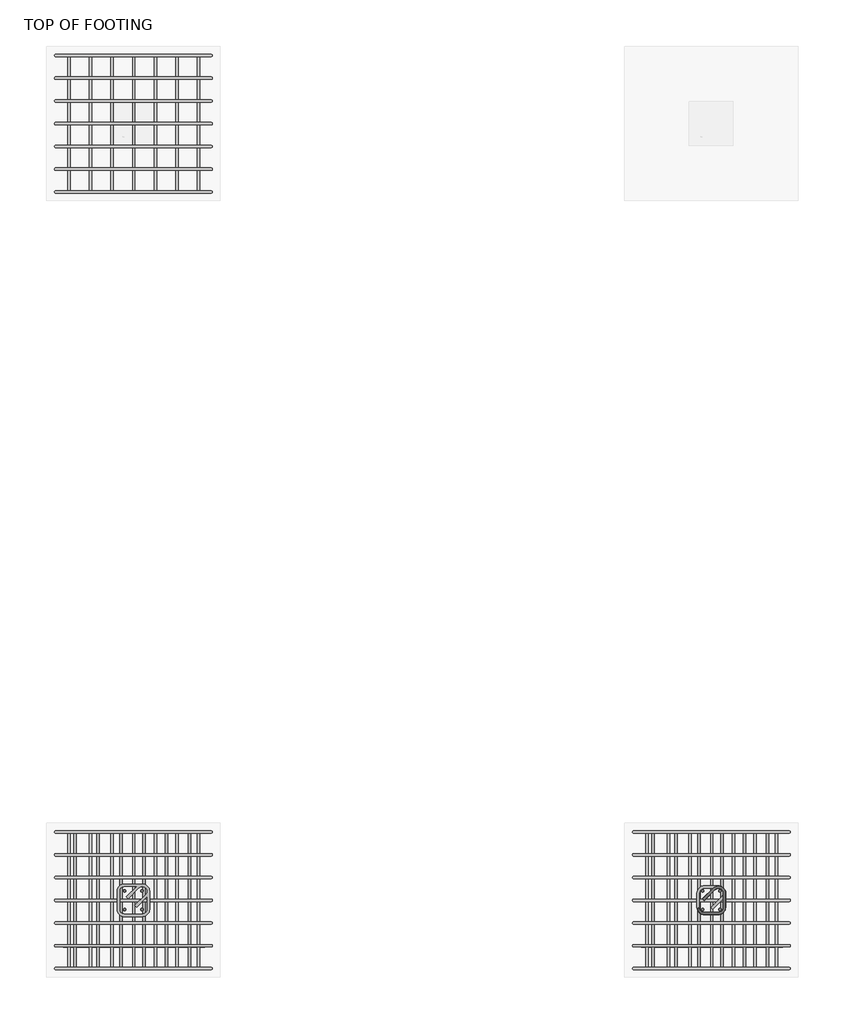
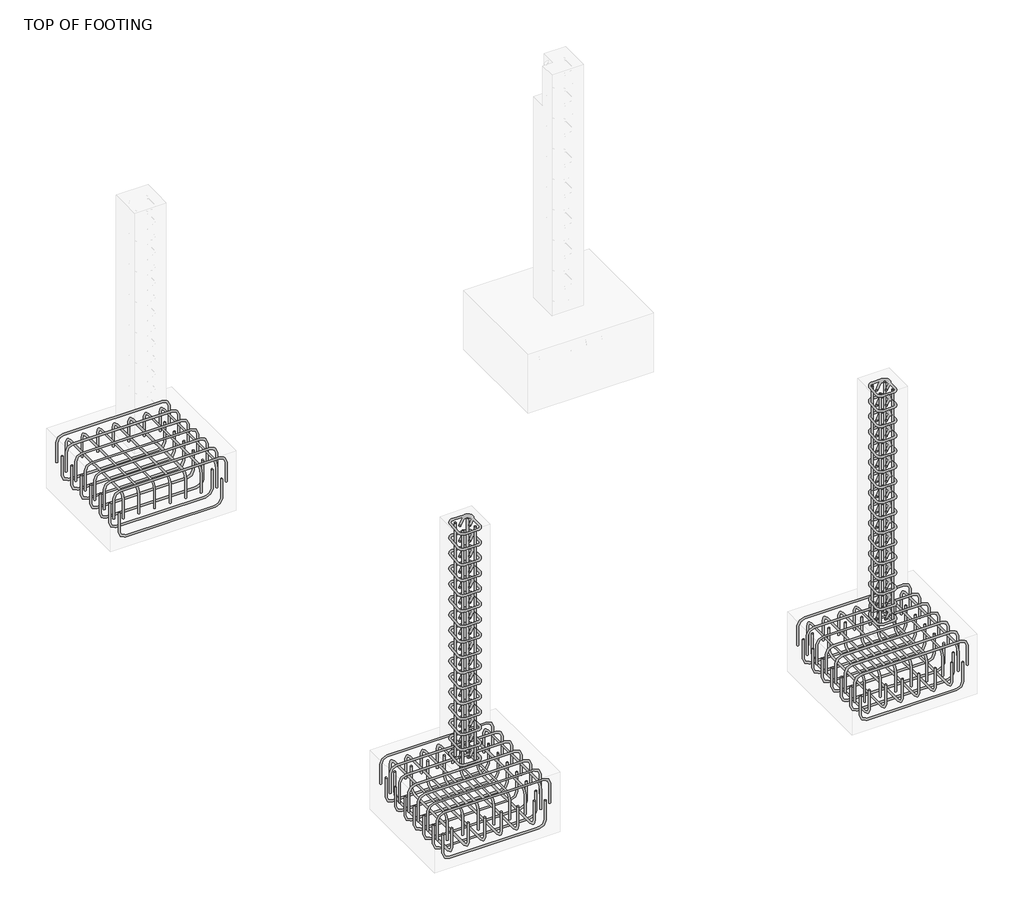
# One storey, part 2 of 6: 17 reinforcing bars.
"""IFC4 building model written with IfcOpenShell, lengths in millimetres."""

from ifc_helpers import new_model, si_unit, point, frame, origin, place, context, project, spatial, polyline, circle_curve, trimmed, segment, composite_curve, source, transform, mapped, element, save
from ifc_brep_helpers import swept_disk

model = new_model("IFC4")

# Units and contexts
model_context = context("Model", 3, world=origin())
ifc_project = project(units=[si_unit("LENGTHUNIT", "METRE", prefix="MILLI")], contexts=[model_context])

# Site, building, storey
site = spatial("IfcSite", under=ifc_project)
building = spatial("IfcBuilding", under=site)
storey = spatial("IfcBuildingStorey", under=building, Name="TOP OF FOOTING", Elevation=-1828.8)

# Reinforcing bars
placement = place(None, origin())
reinforcing_bar_shape = source(origin(), model_context, "Body", "SolidModel", [
    swept_disk(composite_curve([segment(polyline([(-14552.1855212, 120.9474721, -2038.8), (-14552.1855212, 120.9474721, -2186.1)]), True, "CONTINUOUS"), segment(trimmed(circle_curve(frame((-14598.5355212, 120.9474721, -2186.1), z_axis=(0.0, 1.0, 0.0), x_axis=(46.350000000000364, 0.0, 0.0)), 46.35), [point((-14552.1855212, 120.9474721, -2186.1))], [point((-14598.5355212, 120.9474721, -2232.45))], True, "CARTESIAN"), True, "CONTINUOUS"), segment(polyline([(-14598.5355212, 120.9474721, -2232.45), (-15241.6761323, 120.9474721, -2232.45)]), True, "CONTINUOUS"), segment(trimmed(circle_curve(frame((-15241.6761323, 120.9474721, -2186.1), z_axis=(0.0, 1.0, 0.0), x_axis=(0.0, 0.0, -46.34999999999991)), 46.35), [point((-15241.6761323, 120.9474721, -2232.45))], [point((-15288.0261323, 120.9474721, -2186.1))], True, "CARTESIAN"), True, "CONTINUOUS"), segment(polyline([(-15288.0261323, 120.9474721, -2186.1), (-15288.0261323, 120.9474721, -2038.8)]), True, "CONTINUOUS")], self_intersect=False), 6.35),
])
element("IfcReinforcingBar", 1, at=placement, inside=storey, context=model_context, shape_type="MappedRepresentation", body=[
    mapped(reinforcing_bar_shape, transform((0.0, 0.0, 0.0), x_axis=(1.0, 0.0, 0.0), y_axis=(0.0, 1.0, 0.0), z_axis=(0.0, 0.0, 1.0))),
    mapped(reinforcing_bar_shape, transform((0.0, -117.8833333, 0.0), x_axis=(1.0, 0.0, 0.0), y_axis=(0.0, 1.0, 0.0), z_axis=(0.0, 0.0, 1.0))),
    mapped(reinforcing_bar_shape, transform((0.0, -235.7666667, 0.0), x_axis=(1.0, 0.0, 0.0), y_axis=(0.0, 1.0, 0.0), z_axis=(0.0, 0.0, 1.0))),
    mapped(reinforcing_bar_shape, transform((0.0, -353.65, 0.0), x_axis=(1.0, 0.0, 0.0), y_axis=(0.0, 1.0, 0.0), z_axis=(0.0, 0.0, 1.0))),
    mapped(reinforcing_bar_shape, transform((0.0, -471.5333333, 0.0), x_axis=(1.0, 0.0, 0.0), y_axis=(0.0, 1.0, 0.0), z_axis=(0.0, 0.0, 1.0))),
    mapped(reinforcing_bar_shape, transform((0.0, -589.4166667, 0.0), x_axis=(1.0, 0.0, 0.0), y_axis=(0.0, 1.0, 0.0), z_axis=(0.0, 0.0, 1.0))),
    mapped(reinforcing_bar_shape, transform((0.0, -707.3, 0.0), x_axis=(1.0, 0.0, 0.0), y_axis=(0.0, 1.0, 0.0), z_axis=(0.0, 0.0, 1.0))),
])
reinforcing_bar_2_shape = source(origin(), model_context, "Body", "SolidModel", [
    swept_disk(composite_curve([segment(polyline([(-15327.4056799, 120.9474721, -2070.9463075), (-15327.4056799, 120.9474721, -1923.6463075)]), True, "CONTINUOUS"), segment(trimmed(circle_curve(frame((-15281.0556799, 120.9474721, -1923.6463075), z_axis=(0.0, 1.0, 0.0), x_axis=(-46.350000000000364, 0.0, 0.0)), 46.35), [point((-15327.4056799, 120.9474721, -1923.6463075))], [point((-15281.0556799, 120.9474721, -1877.2963075))], True, "CARTESIAN"), True, "CONTINUOUS"), segment(polyline([(-15281.0556799, 120.9474721, -1877.2963075), (-14566.4556799, 120.9474721, -1877.2963075)]), True, "CONTINUOUS"), segment(trimmed(circle_curve(frame((-14566.4556799, 120.9474721, -1923.6463075), z_axis=(0.0, 1.0, 0.0), x_axis=(0.0, 0.0, 46.34999999999991)), 46.35), [point((-14566.4556799, 120.9474721, -1877.2963075))], [point((-14520.1056799, 120.9474721, -1923.6463075))], True, "CARTESIAN"), True, "CONTINUOUS"), segment(polyline([(-14520.1056799, 120.9474721, -1923.6463075), (-14520.1056799, 120.9474721, -2070.9463075)]), True, "CONTINUOUS")], self_intersect=False), 6.35),
])
element("IfcReinforcingBar", 2, at=placement, inside=storey, context=model_context, shape_type="MappedRepresentation", body=[
    mapped(reinforcing_bar_2_shape, transform((0.0, 0.0, 0.0), x_axis=(1.0, 0.0, 0.0), y_axis=(0.0, 1.0, 0.0), z_axis=(0.0, 0.0, 1.0))),
    mapped(reinforcing_bar_2_shape, transform((0.0, -117.8833333, 0.0), x_axis=(1.0, 0.0, 0.0), y_axis=(0.0, 1.0, 0.0), z_axis=(0.0, 0.0, 1.0))),
    mapped(reinforcing_bar_2_shape, transform((0.0, -235.7666667, 0.0), x_axis=(1.0, 0.0, 0.0), y_axis=(0.0, 1.0, 0.0), z_axis=(0.0, 0.0, 1.0))),
    mapped(reinforcing_bar_2_shape, transform((0.0, -353.65, 0.0), x_axis=(1.0, 0.0, 0.0), y_axis=(0.0, 1.0, 0.0), z_axis=(0.0, 0.0, 1.0))),
    mapped(reinforcing_bar_2_shape, transform((0.0, -471.5333333, 0.0), x_axis=(1.0, 0.0, 0.0), y_axis=(0.0, 1.0, 0.0), z_axis=(0.0, 0.0, 1.0))),
    mapped(reinforcing_bar_2_shape, transform((0.0, -589.4166667, 0.0), x_axis=(1.0, 0.0, 0.0), y_axis=(0.0, 1.0, 0.0), z_axis=(0.0, 0.0, 1.0))),
    mapped(reinforcing_bar_2_shape, transform((0.0, -707.3, 0.0), x_axis=(1.0, 0.0, 0.0), y_axis=(0.0, 1.0, 0.0), z_axis=(0.0, 0.0, 1.0))),
])
reinforcing_bar_3_shape = source(origin(), model_context, "Body", "SolidModel", [
    swept_disk(composite_curve([segment(polyline([(-14585.2545962, 120.9474721, -2094.0228735), (-14585.2545962, 120.9474721, -1946.7228735)]), True, "CONTINUOUS"), segment(trimmed(circle_curve(frame((-14585.2545962, 74.5974721, -1946.7228735), z_axis=(1.0, 0.0, 0.0), x_axis=(0.0, 46.349999999999994, 0.0)), 46.35), [point((-14585.2545962, 120.9474721, -1946.7228735))], [point((-14585.2545962, 74.5974721, -1900.3728735))], True, "CARTESIAN"), True, "CONTINUOUS"), segment(polyline([(-14585.2545962, 74.5974721, -1900.3728735), (-14585.2545962, -540.0025279, -1900.3728735)]), True, "CONTINUOUS"), segment(trimmed(circle_curve(frame((-14585.2545962, -540.0025279, -1946.7228735), z_axis=(1.0, 0.0, 0.0), x_axis=(0.0, 0.0, 46.350000000000136)), 46.35), [point((-14585.2545962, -540.0025279, -1900.3728735))], [point((-14585.2545962, -586.3525279, -1946.7228735))], True, "CARTESIAN"), True, "CONTINUOUS"), segment(polyline([(-14585.2545962, -586.3525279, -1946.7228735), (-14585.2545962, -586.3525279, -2094.0228735)]), True, "CONTINUOUS")], self_intersect=False), 6.35),
])
element("IfcReinforcingBar", 3, at=placement, inside=storey, context=model_context, shape_type="MappedRepresentation", body=[
    mapped(reinforcing_bar_3_shape, transform((0.0, 0.0, 0.0), x_axis=(1.0, 0.0, 0.0), y_axis=(0.0, 1.0, 0.0), z_axis=(0.0, 0.0, 1.0))),
    mapped(reinforcing_bar_3_shape, transform((-112.124631, 0.0, 0.0), x_axis=(1.0, 0.0, 0.0), y_axis=(0.0, 1.0, 0.0), z_axis=(0.0, 0.0, 1.0))),
    mapped(reinforcing_bar_3_shape, transform((-224.2492621, 0.0, 0.0), x_axis=(1.0, 0.0, 0.0), y_axis=(0.0, 1.0, 0.0), z_axis=(0.0, 0.0, 1.0))),
    mapped(reinforcing_bar_3_shape, transform((-336.3738931, 0.0, 0.0), x_axis=(1.0, 0.0, 0.0), y_axis=(0.0, 1.0, 0.0), z_axis=(0.0, 0.0, 1.0))),
    mapped(reinforcing_bar_3_shape, transform((-448.4985241, 0.0, 0.0), x_axis=(1.0, 0.0, 0.0), y_axis=(0.0, 1.0, 0.0), z_axis=(0.0, 0.0, 1.0))),
    mapped(reinforcing_bar_3_shape, transform((-560.6231552, 0.0, 0.0), x_axis=(1.0, 0.0, 0.0), y_axis=(0.0, 1.0, 0.0), z_axis=(0.0, 0.0, 1.0))),
    mapped(reinforcing_bar_3_shape, transform((-672.7477862, 0.0, 0.0), x_axis=(1.0, 0.0, 0.0), y_axis=(0.0, 1.0, 0.0), z_axis=(0.0, 0.0, 1.0))),
])
reinforcing_bar_4_shape = source(origin(), model_context, "Body", "SolidModel", [
    swept_disk(composite_curve([segment(polyline([(-14552.1855212, -3906.2483349, -2038.8), (-14552.1855212, -3906.2483349, -2186.1)]), True, "CONTINUOUS"), segment(trimmed(circle_curve(frame((-14598.5355212, -3906.2483349, -2186.1), z_axis=(0.0, 1.0, 0.0), x_axis=(46.350000000000364, 0.0, 0.0)), 46.35), [point((-14552.1855212, -3906.2483349, -2186.1))], [point((-14598.5355212, -3906.2483349, -2232.45))], True, "CARTESIAN"), True, "CONTINUOUS"), segment(polyline([(-14598.5355212, -3906.2483349, -2232.45), (-15241.6761323, -3906.2483349, -2232.45)]), True, "CONTINUOUS"), segment(trimmed(circle_curve(frame((-15241.6761323, -3906.2483349, -2186.1), z_axis=(0.0, 1.0, 0.0), x_axis=(0.0, 0.0, -46.34999999999991)), 46.35), [point((-15241.6761323, -3906.2483349, -2232.45))], [point((-15288.0261323, -3906.2483349, -2186.1))], True, "CARTESIAN"), True, "CONTINUOUS"), segment(polyline([(-15288.0261323, -3906.2483349, -2186.1), (-15288.0261323, -3906.2483349, -2038.8)]), True, "CONTINUOUS")], self_intersect=False), 6.35),
])
element("IfcReinforcingBar", 4, at=placement, inside=storey, context=model_context, shape_type="MappedRepresentation", body=[
    mapped(reinforcing_bar_4_shape, transform((0.0, 0.0, 0.0), x_axis=(1.0, 0.0, 0.0), y_axis=(0.0, 1.0, 0.0), z_axis=(0.0, 0.0, 1.0))),
    mapped(reinforcing_bar_4_shape, transform((0.0, -117.8833333, 0.0), x_axis=(1.0, 0.0, 0.0), y_axis=(0.0, 1.0, 0.0), z_axis=(0.0, 0.0, 1.0))),
    mapped(reinforcing_bar_4_shape, transform((0.0, -235.7666667, 0.0), x_axis=(1.0, 0.0, 0.0), y_axis=(0.0, 1.0, 0.0), z_axis=(0.0, 0.0, 1.0))),
    mapped(reinforcing_bar_4_shape, transform((0.0, -353.65, 0.0), x_axis=(1.0, 0.0, 0.0), y_axis=(0.0, 1.0, 0.0), z_axis=(0.0, 0.0, 1.0))),
    mapped(reinforcing_bar_4_shape, transform((0.0, -471.5333333, 0.0), x_axis=(1.0, 0.0, 0.0), y_axis=(0.0, 1.0, 0.0), z_axis=(0.0, 0.0, 1.0))),
    mapped(reinforcing_bar_4_shape, transform((0.0, -589.4166667, 0.0), x_axis=(1.0, 0.0, 0.0), y_axis=(0.0, 1.0, 0.0), z_axis=(0.0, 0.0, 1.0))),
    mapped(reinforcing_bar_4_shape, transform((0.0, -707.3, 0.0), x_axis=(1.0, 0.0, 0.0), y_axis=(0.0, 1.0, 0.0), z_axis=(0.0, 0.0, 1.0))),
])
reinforcing_bar_5_shape = source(origin(), model_context, "Body", "SolidModel", [
    swept_disk(composite_curve([segment(polyline([(-15327.4056799, -3906.2483349, -2070.9463075), (-15327.4056799, -3906.2483349, -1923.6463075)]), True, "CONTINUOUS"), segment(trimmed(circle_curve(frame((-15281.0556799, -3906.2483349, -1923.6463075), z_axis=(0.0, 1.0, 0.0), x_axis=(-46.350000000000364, 0.0, 0.0)), 46.35), [point((-15327.4056799, -3906.2483349, -1923.6463075))], [point((-15281.0556799, -3906.2483349, -1877.2963075))], True, "CARTESIAN"), True, "CONTINUOUS"), segment(polyline([(-15281.0556799, -3906.2483349, -1877.2963075), (-14566.4556799, -3906.2483349, -1877.2963075)]), True, "CONTINUOUS"), segment(trimmed(circle_curve(frame((-14566.4556799, -3906.2483349, -1923.6463075), z_axis=(0.0, 1.0, 0.0), x_axis=(0.0, 0.0, 46.34999999999991)), 46.35), [point((-14566.4556799, -3906.2483349, -1877.2963075))], [point((-14520.1056799, -3906.2483349, -1923.6463075))], True, "CARTESIAN"), True, "CONTINUOUS"), segment(polyline([(-14520.1056799, -3906.2483349, -1923.6463075), (-14520.1056799, -3906.2483349, -2070.9463075)]), True, "CONTINUOUS")], self_intersect=False), 6.35),
])
element("IfcReinforcingBar", 5, at=placement, inside=storey, context=model_context, shape_type="MappedRepresentation", body=[
    mapped(reinforcing_bar_5_shape, transform((0.0, 0.0, 0.0), x_axis=(1.0, 0.0, 0.0), y_axis=(0.0, 1.0, 0.0), z_axis=(0.0, 0.0, 1.0))),
    mapped(reinforcing_bar_5_shape, transform((0.0, -117.8833333, 0.0), x_axis=(1.0, 0.0, 0.0), y_axis=(0.0, 1.0, 0.0), z_axis=(0.0, 0.0, 1.0))),
    mapped(reinforcing_bar_5_shape, transform((0.0, -235.7666667, 0.0), x_axis=(1.0, 0.0, 0.0), y_axis=(0.0, 1.0, 0.0), z_axis=(0.0, 0.0, 1.0))),
    mapped(reinforcing_bar_5_shape, transform((0.0, -353.65, 0.0), x_axis=(1.0, 0.0, 0.0), y_axis=(0.0, 1.0, 0.0), z_axis=(0.0, 0.0, 1.0))),
    mapped(reinforcing_bar_5_shape, transform((0.0, -471.5333333, 0.0), x_axis=(1.0, 0.0, 0.0), y_axis=(0.0, 1.0, 0.0), z_axis=(0.0, 0.0, 1.0))),
    mapped(reinforcing_bar_5_shape, transform((0.0, -589.4166667, 0.0), x_axis=(1.0, 0.0, 0.0), y_axis=(0.0, 1.0, 0.0), z_axis=(0.0, 0.0, 1.0))),
    mapped(reinforcing_bar_5_shape, transform((0.0, -707.3, 0.0), x_axis=(1.0, 0.0, 0.0), y_axis=(0.0, 1.0, 0.0), z_axis=(0.0, 0.0, 1.0))),
])
reinforcing_bar_6_shape = source(origin(), model_context, "Body", "SolidModel", [
    swept_disk(composite_curve([segment(polyline([(-14585.2545962, -3906.2483349, -2094.0228735), (-14585.2545962, -3906.2483349, -1946.7228735)]), True, "CONTINUOUS"), segment(trimmed(circle_curve(frame((-14585.2545962, -3952.5983349, -1946.7228735), z_axis=(1.0, 0.0, 0.0), x_axis=(0.0, 46.34999999999991, 0.0)), 46.35), [point((-14585.2545962, -3906.2483349, -1946.7228735))], [point((-14585.2545962, -3952.5983349, -1900.3728735))], True, "CARTESIAN"), True, "CONTINUOUS"), segment(polyline([(-14585.2545962, -3952.5983349, -1900.3728735), (-14585.2545962, -4567.1983349, -1900.3728735)]), True, "CONTINUOUS"), segment(trimmed(circle_curve(frame((-14585.2545962, -4567.1983349, -1946.7228735), z_axis=(1.0, 0.0, 0.0), x_axis=(0.0, 0.0, 46.350000000000136)), 46.35), [point((-14585.2545962, -4567.1983349, -1900.3728735))], [point((-14585.2545962, -4613.5483349, -1946.7228735))], True, "CARTESIAN"), True, "CONTINUOUS"), segment(polyline([(-14585.2545962, -4613.5483349, -1946.7228735), (-14585.2545962, -4613.5483349, -2094.0228735)]), True, "CONTINUOUS")], self_intersect=False), 6.35),
])
element("IfcReinforcingBar", 6, at=placement, inside=storey, context=model_context, shape_type="MappedRepresentation", body=[
    mapped(reinforcing_bar_6_shape, transform((0.0, 0.0, 0.0), x_axis=(1.0, 0.0, 0.0), y_axis=(0.0, 1.0, 0.0), z_axis=(0.0, 0.0, 1.0))),
    mapped(reinforcing_bar_6_shape, transform((-112.124631, 0.0, 0.0), x_axis=(1.0, 0.0, 0.0), y_axis=(0.0, 1.0, 0.0), z_axis=(0.0, 0.0, 1.0))),
    mapped(reinforcing_bar_6_shape, transform((-224.2492621, 0.0, 0.0), x_axis=(1.0, 0.0, 0.0), y_axis=(0.0, 1.0, 0.0), z_axis=(0.0, 0.0, 1.0))),
    mapped(reinforcing_bar_6_shape, transform((-336.3738931, 0.0, 0.0), x_axis=(1.0, 0.0, 0.0), y_axis=(0.0, 1.0, 0.0), z_axis=(0.0, 0.0, 1.0))),
    mapped(reinforcing_bar_6_shape, transform((-448.4985241, 0.0, 0.0), x_axis=(1.0, 0.0, 0.0), y_axis=(0.0, 1.0, 0.0), z_axis=(0.0, 0.0, 1.0))),
    mapped(reinforcing_bar_6_shape, transform((-560.6231552, 0.0, 0.0), x_axis=(1.0, 0.0, 0.0), y_axis=(0.0, 1.0, 0.0), z_axis=(0.0, 0.0, 1.0))),
    mapped(reinforcing_bar_6_shape, transform((-672.7477862, 0.0, 0.0), x_axis=(1.0, 0.0, 0.0), y_axis=(0.0, 1.0, 0.0), z_axis=(0.0, 0.0, 1.0))),
])
reinforcing_bar_7_shape = source(origin(), model_context, "Body", "SolidModel", [
    swept_disk(composite_curve([segment(polyline([(-15225.2448384, -3906.2483349, -2014.7438142), (-15225.2448384, -3906.2483349, -2162.0438142)]), True, "CONTINUOUS"), segment(trimmed(circle_curve(frame((-15225.2448384, -3952.5983349, -2162.0438142), z_axis=(-1.0, 0.0, 0.0), x_axis=(0.0, 46.34999999999991, 0.0)), 46.35), [point((-15225.2448384, -3906.2483349, -2162.0438142))], [point((-15225.2448384, -3952.5983349, -2208.3938142))], True, "CARTESIAN"), True, "CONTINUOUS"), segment(polyline([(-15225.2448384, -3952.5983349, -2208.3938142), (-15225.2448384, -4567.1983349, -2208.3938142)]), True, "CONTINUOUS"), segment(trimmed(circle_curve(frame((-15225.2448384, -4567.1983349, -2162.0438142), z_axis=(-1.0, 0.0, 0.0), x_axis=(0.0, 0.0, -46.350000000000364)), 46.35), [point((-15225.2448384, -4567.1983349, -2208.3938142))], [point((-15225.2448384, -4613.5483349, -2162.0438142))], True, "CARTESIAN"), True, "CONTINUOUS"), segment(polyline([(-15225.2448384, -4613.5483349, -2162.0438142), (-15225.2448384, -4613.5483349, -2014.7438142)]), True, "CONTINUOUS")], self_intersect=False), 6.35),
])
element("IfcReinforcingBar", 7, at=placement, inside=storey, context=model_context, shape_type="MappedRepresentation", body=[
    mapped(reinforcing_bar_7_shape, transform((0.0, 0.0, 0.0), x_axis=(1.0, 0.0, 0.0), y_axis=(0.0, 1.0, 0.0), z_axis=(0.0, 0.0, 1.0))),
    mapped(reinforcing_bar_7_shape, transform((118.647936, 0.0, 0.0), x_axis=(1.0, 0.0, 0.0), y_axis=(0.0, 1.0, 0.0), z_axis=(0.0, 0.0, 1.0))),
    mapped(reinforcing_bar_7_shape, transform((237.295872, 0.0, 0.0), x_axis=(1.0, 0.0, 0.0), y_axis=(0.0, 1.0, 0.0), z_axis=(0.0, 0.0, 1.0))),
    mapped(reinforcing_bar_7_shape, transform((355.943808, 0.0, 0.0), x_axis=(1.0, 0.0, 0.0), y_axis=(0.0, 1.0, 0.0), z_axis=(0.0, 0.0, 1.0))),
    mapped(reinforcing_bar_7_shape, transform((474.591744, 0.0, 0.0), x_axis=(1.0, 0.0, 0.0), y_axis=(0.0, 1.0, 0.0), z_axis=(0.0, 0.0, 1.0))),
    mapped(reinforcing_bar_7_shape, transform((593.23968, 0.0, 0.0), x_axis=(1.0, 0.0, 0.0), y_axis=(0.0, 1.0, 0.0), z_axis=(0.0, 0.0, 1.0))),
])
reinforcing_bar_8_shape = source(origin(), model_context, "Body", "SolidModel", [
    swept_disk(composite_curve([segment(polyline([(-11554.9855212, -3906.2483349, -2038.8), (-11554.9855212, -3906.2483349, -2186.1)]), True, "CONTINUOUS"), segment(trimmed(circle_curve(frame((-11601.3355212, -3906.2483349, -2186.1), z_axis=(0.0, 1.0, 0.0), x_axis=(46.350000000000364, 0.0, 0.0)), 46.35), [point((-11554.9855212, -3906.2483349, -2186.1))], [point((-11601.3355212, -3906.2483349, -2232.45))], True, "CARTESIAN"), True, "CONTINUOUS"), segment(polyline([(-11601.3355212, -3906.2483349, -2232.45), (-12244.4761323, -3906.2483349, -2232.45)]), True, "CONTINUOUS"), segment(trimmed(circle_curve(frame((-12244.4761323, -3906.2483349, -2186.1), z_axis=(0.0, 1.0, 0.0), x_axis=(0.0, 0.0, -46.34999999999991)), 46.35), [point((-12244.4761323, -3906.2483349, -2232.45))], [point((-12290.8261323, -3906.2483349, -2186.1))], True, "CARTESIAN"), True, "CONTINUOUS"), segment(polyline([(-12290.8261323, -3906.2483349, -2186.1), (-12290.8261323, -3906.2483349, -2038.8)]), True, "CONTINUOUS")], self_intersect=False), 6.35),
])
element("IfcReinforcingBar", 8, at=placement, inside=storey, context=model_context, shape_type="MappedRepresentation", body=[
    mapped(reinforcing_bar_8_shape, transform((0.0, 0.0, 0.0), x_axis=(1.0, 0.0, 0.0), y_axis=(0.0, 1.0, 0.0), z_axis=(0.0, 0.0, 1.0))),
    mapped(reinforcing_bar_8_shape, transform((0.0, -117.8833333, 0.0), x_axis=(1.0, 0.0, 0.0), y_axis=(0.0, 1.0, 0.0), z_axis=(0.0, 0.0, 1.0))),
    mapped(reinforcing_bar_8_shape, transform((0.0, -235.7666667, 0.0), x_axis=(1.0, 0.0, 0.0), y_axis=(0.0, 1.0, 0.0), z_axis=(0.0, 0.0, 1.0))),
    mapped(reinforcing_bar_8_shape, transform((0.0, -353.65, 0.0), x_axis=(1.0, 0.0, 0.0), y_axis=(0.0, 1.0, 0.0), z_axis=(0.0, 0.0, 1.0))),
    mapped(reinforcing_bar_8_shape, transform((0.0, -471.5333333, 0.0), x_axis=(1.0, 0.0, 0.0), y_axis=(0.0, 1.0, 0.0), z_axis=(0.0, 0.0, 1.0))),
    mapped(reinforcing_bar_8_shape, transform((0.0, -589.4166667, 0.0), x_axis=(1.0, 0.0, 0.0), y_axis=(0.0, 1.0, 0.0), z_axis=(0.0, 0.0, 1.0))),
    mapped(reinforcing_bar_8_shape, transform((0.0, -707.3, 0.0), x_axis=(1.0, 0.0, 0.0), y_axis=(0.0, 1.0, 0.0), z_axis=(0.0, 0.0, 1.0))),
])
reinforcing_bar_9_shape = source(origin(), model_context, "Body", "SolidModel", [
    swept_disk(composite_curve([segment(polyline([(-12330.2056799, -3906.2483349, -2070.9463075), (-12330.2056799, -3906.2483349, -1923.6463075)]), True, "CONTINUOUS"), segment(trimmed(circle_curve(frame((-12283.8556799, -3906.2483349, -1923.6463075), z_axis=(0.0, 1.0, 0.0), x_axis=(-46.350000000000364, 0.0, 0.0)), 46.35), [point((-12330.2056799, -3906.2483349, -1923.6463075))], [point((-12283.8556799, -3906.2483349, -1877.2963075))], True, "CARTESIAN"), True, "CONTINUOUS"), segment(polyline([(-12283.8556799, -3906.2483349, -1877.2963075), (-11569.2556799, -3906.2483349, -1877.2963075)]), True, "CONTINUOUS"), segment(trimmed(circle_curve(frame((-11569.2556799, -3906.2483349, -1923.6463075), z_axis=(0.0, 1.0, 0.0), x_axis=(0.0, 0.0, 46.34999999999991)), 46.35), [point((-11569.2556799, -3906.2483349, -1877.2963075))], [point((-11522.9056799, -3906.2483349, -1923.6463075))], True, "CARTESIAN"), True, "CONTINUOUS"), segment(polyline([(-11522.9056799, -3906.2483349, -1923.6463075), (-11522.9056799, -3906.2483349, -2070.9463075)]), True, "CONTINUOUS")], self_intersect=False), 6.35),
])
element("IfcReinforcingBar", 9, at=placement, inside=storey, context=model_context, shape_type="MappedRepresentation", body=[
    mapped(reinforcing_bar_9_shape, transform((0.0, 0.0, 0.0), x_axis=(1.0, 0.0, 0.0), y_axis=(0.0, 1.0, 0.0), z_axis=(0.0, 0.0, 1.0))),
    mapped(reinforcing_bar_9_shape, transform((0.0, -117.8833333, 0.0), x_axis=(1.0, 0.0, 0.0), y_axis=(0.0, 1.0, 0.0), z_axis=(0.0, 0.0, 1.0))),
    mapped(reinforcing_bar_9_shape, transform((0.0, -235.7666667, 0.0), x_axis=(1.0, 0.0, 0.0), y_axis=(0.0, 1.0, 0.0), z_axis=(0.0, 0.0, 1.0))),
    mapped(reinforcing_bar_9_shape, transform((0.0, -353.65, 0.0), x_axis=(1.0, 0.0, 0.0), y_axis=(0.0, 1.0, 0.0), z_axis=(0.0, 0.0, 1.0))),
    mapped(reinforcing_bar_9_shape, transform((0.0, -471.5333333, 0.0), x_axis=(1.0, 0.0, 0.0), y_axis=(0.0, 1.0, 0.0), z_axis=(0.0, 0.0, 1.0))),
    mapped(reinforcing_bar_9_shape, transform((0.0, -589.4166667, 0.0), x_axis=(1.0, 0.0, 0.0), y_axis=(0.0, 1.0, 0.0), z_axis=(0.0, 0.0, 1.0))),
    mapped(reinforcing_bar_9_shape, transform((0.0, -707.3, 0.0), x_axis=(1.0, 0.0, 0.0), y_axis=(0.0, 1.0, 0.0), z_axis=(0.0, 0.0, 1.0))),
])
reinforcing_bar_10_shape = source(origin(), model_context, "Body", "SolidModel", [
    swept_disk(composite_curve([segment(polyline([(-11588.0545962, -3906.2483349, -2094.0228735), (-11588.0545962, -3906.2483349, -1946.7228735)]), True, "CONTINUOUS"), segment(trimmed(circle_curve(frame((-11588.0545962, -3952.5983349, -1946.7228735), z_axis=(1.0, 0.0, 0.0), x_axis=(0.0, 46.34999999999991, 0.0)), 46.35), [point((-11588.0545962, -3906.2483349, -1946.7228735))], [point((-11588.0545962, -3952.5983349, -1900.3728735))], True, "CARTESIAN"), True, "CONTINUOUS"), segment(polyline([(-11588.0545962, -3952.5983349, -1900.3728735), (-11588.0545962, -4567.1983349, -1900.3728735)]), True, "CONTINUOUS"), segment(trimmed(circle_curve(frame((-11588.0545962, -4567.1983349, -1946.7228735), z_axis=(1.0, 0.0, 0.0), x_axis=(0.0, 0.0, 46.350000000000136)), 46.35), [point((-11588.0545962, -4567.1983349, -1900.3728735))], [point((-11588.0545962, -4613.5483349, -1946.7228735))], True, "CARTESIAN"), True, "CONTINUOUS"), segment(polyline([(-11588.0545962, -4613.5483349, -1946.7228735), (-11588.0545962, -4613.5483349, -2094.0228735)]), True, "CONTINUOUS")], self_intersect=False), 6.35),
])
element("IfcReinforcingBar", 10, at=placement, inside=storey, context=model_context, shape_type="MappedRepresentation", body=[
    mapped(reinforcing_bar_10_shape, transform((0.0, 0.0, 0.0), x_axis=(1.0, 0.0, 0.0), y_axis=(0.0, 1.0, 0.0), z_axis=(0.0, 0.0, 1.0))),
    mapped(reinforcing_bar_10_shape, transform((-112.124631, 0.0, 0.0), x_axis=(1.0, 0.0, 0.0), y_axis=(0.0, 1.0, 0.0), z_axis=(0.0, 0.0, 1.0))),
    mapped(reinforcing_bar_10_shape, transform((-224.2492621, 0.0, 0.0), x_axis=(1.0, 0.0, 0.0), y_axis=(0.0, 1.0, 0.0), z_axis=(0.0, 0.0, 1.0))),
    mapped(reinforcing_bar_10_shape, transform((-336.3738931, 0.0, 0.0), x_axis=(1.0, 0.0, 0.0), y_axis=(0.0, 1.0, 0.0), z_axis=(0.0, 0.0, 1.0))),
    mapped(reinforcing_bar_10_shape, transform((-448.4985241, 0.0, 0.0), x_axis=(1.0, 0.0, 0.0), y_axis=(0.0, 1.0, 0.0), z_axis=(0.0, 0.0, 1.0))),
    mapped(reinforcing_bar_10_shape, transform((-560.6231552, 0.0, 0.0), x_axis=(1.0, 0.0, 0.0), y_axis=(0.0, 1.0, 0.0), z_axis=(0.0, 0.0, 1.0))),
    mapped(reinforcing_bar_10_shape, transform((-672.7477862, 0.0, 0.0), x_axis=(1.0, 0.0, 0.0), y_axis=(0.0, 1.0, 0.0), z_axis=(0.0, 0.0, 1.0))),
])
reinforcing_bar_11_shape = source(origin(), model_context, "Body", "SolidModel", [
    swept_disk(composite_curve([segment(polyline([(-12228.0448384, -3906.2483349, -2014.7438142), (-12228.0448384, -3906.2483349, -2162.0438142)]), True, "CONTINUOUS"), segment(trimmed(circle_curve(frame((-12228.0448384, -3952.5983349, -2162.0438142), z_axis=(-1.0, 0.0, 0.0), x_axis=(0.0, 46.34999999999991, 0.0)), 46.35), [point((-12228.0448384, -3906.2483349, -2162.0438142))], [point((-12228.0448384, -3952.5983349, -2208.3938142))], True, "CARTESIAN"), True, "CONTINUOUS"), segment(polyline([(-12228.0448384, -3952.5983349, -2208.3938142), (-12228.0448384, -4567.1983349, -2208.3938142)]), True, "CONTINUOUS"), segment(trimmed(circle_curve(frame((-12228.0448384, -4567.1983349, -2162.0438142), z_axis=(-1.0, 0.0, 0.0), x_axis=(0.0, 0.0, -46.350000000000364)), 46.35), [point((-12228.0448384, -4567.1983349, -2208.3938142))], [point((-12228.0448384, -4613.5483349, -2162.0438142))], True, "CARTESIAN"), True, "CONTINUOUS"), segment(polyline([(-12228.0448384, -4613.5483349, -2162.0438142), (-12228.0448384, -4613.5483349, -2014.7438142)]), True, "CONTINUOUS")], self_intersect=False), 6.35),
])
element("IfcReinforcingBar", 11, at=placement, inside=storey, context=model_context, shape_type="MappedRepresentation", body=[
    mapped(reinforcing_bar_11_shape, transform((0.0, 0.0, 0.0), x_axis=(1.0, 0.0, 0.0), y_axis=(0.0, 1.0, 0.0), z_axis=(0.0, 0.0, 1.0))),
    mapped(reinforcing_bar_11_shape, transform((118.647936, 0.0, 0.0), x_axis=(1.0, 0.0, 0.0), y_axis=(0.0, 1.0, 0.0), z_axis=(0.0, 0.0, 1.0))),
    mapped(reinforcing_bar_11_shape, transform((237.295872, 0.0, 0.0), x_axis=(1.0, 0.0, 0.0), y_axis=(0.0, 1.0, 0.0), z_axis=(0.0, 0.0, 1.0))),
    mapped(reinforcing_bar_11_shape, transform((355.943808, 0.0, 0.0), x_axis=(1.0, 0.0, 0.0), y_axis=(0.0, 1.0, 0.0), z_axis=(0.0, 0.0, 1.0))),
    mapped(reinforcing_bar_11_shape, transform((474.591744, 0.0, 0.0), x_axis=(1.0, 0.0, 0.0), y_axis=(0.0, 1.0, 0.0), z_axis=(0.0, 0.0, 1.0))),
    mapped(reinforcing_bar_11_shape, transform((593.23968, 0.0, 0.0), x_axis=(1.0, 0.0, 0.0), y_axis=(0.0, 1.0, 0.0), z_axis=(0.0, 0.0, 1.0))),
])
reinforcing_bar_12_shape = source(origin(), model_context, "Body", "SolidModel", [
    swept_disk(composite_curve([segment(polyline([(-14879.0006936, -4211.1006392, -30.0), (-14879.0006936, -4211.1006392, -1798.8)]), True, "CONTINUOUS")], self_intersect=False), 6.35),
])
element("IfcReinforcingBar", 12, at=placement, inside=storey, context=model_context, shape_type="MappedRepresentation", body=[
    mapped(reinforcing_bar_12_shape, transform((0.0, 0.0, 0.0), x_axis=(1.0, 0.0, 0.0), y_axis=(0.0, 1.0, 0.0), z_axis=(0.0, 0.0, 1.0))),
    mapped(reinforcing_bar_12_shape, transform((0.0, -96.9916148, 0.0), x_axis=(1.0, 0.0, 0.0), y_axis=(0.0, 1.0, 0.0), z_axis=(0.0, 0.0, 1.0))),
])
reinforcing_bar_13_shape = source(origin(), model_context, "Body", "SolidModel", [
    swept_disk(composite_curve([segment(polyline([(-14955.0670404, -4246.8741003, -36.35), (-14899.3234775, -4191.1305373, -36.35)]), True, "CONTINUOUS"), segment(trimmed(circle_curve(frame((-14877.1556799, -4213.2983349, -36.35), z_axis=(0.0, 0.0, -1.0), x_axis=(-22.167797599999176, 22.167797600000085, 0.0)), 31.35), [point((-14899.3234775, -4191.1305373, -36.35))], [point((-14845.8056799, -4213.2983349, -36.35))], True, "CARTESIAN"), True, "CONTINUOUS"), segment(polyline([(-14845.8056799, -4213.2983349, -36.35), (-14845.8056799, -4306.4983349, -36.35)]), True, "CONTINUOUS"), segment(trimmed(circle_curve(frame((-14877.1556799, -4306.4983349, -36.35), z_axis=(0.0, 0.0, -1.0), x_axis=(31.350000000000364, 0.0, 0.0)), 31.35), [point((-14845.8056799, -4306.4983349, -36.35))], [point((-14877.1556799, -4337.8483349, -36.35))], True, "CARTESIAN"), True, "CONTINUOUS"), segment(polyline([(-14877.1556799, -4337.8483349, -36.35), (-14970.3556799, -4337.8483349, -36.35)]), True, "CONTINUOUS"), segment(trimmed(circle_curve(frame((-14970.3556799, -4306.6018415, -33.8045833), z_axis=(0.0, 0.0811935158564889, -0.9966983560650946), x_axis=(0.0, -31.246493399999963, -2.545416700000004)), 31.35), [point((-14970.3556799, -4337.8483349, -36.35))], [point((-15001.7056799, -4306.6018415, -33.8045833))], True, "CARTESIAN"), True, "CONTINUOUS"), segment(polyline([(-15001.7056799, -4306.6018415, -33.8045833), (-15001.7056799, -4213.1948284, -26.1954167)]), True, "CONTINUOUS"), segment(trimmed(circle_curve(frame((-14970.3556799, -4213.1948284, -26.1954167), z_axis=(0.0, 0.0811935158564889, -0.9966983560650946), x_axis=(-31.350000000000364, 0.0, 0.0)), 31.35), [point((-15001.7056799, -4213.1948284, -26.1954167))], [point((-14970.3556799, -4181.9483349, -23.65))], True, "CARTESIAN"), True, "CONTINUOUS"), segment(polyline([(-14970.3556799, -4181.9483349, -23.65), (-14877.1556799, -4181.9483349, -23.65)]), True, "CONTINUOUS"), segment(trimmed(circle_curve(frame((-14877.1556799, -4213.2983349, -23.65), z_axis=(0.0, 0.0, -1.0), x_axis=(0.0, 31.349999999999454, 0.0)), 31.35), [point((-14877.1556799, -4181.9483349, -23.65))], [point((-14854.9878823, -4235.4661325, -23.65))], True, "CARTESIAN"), True, "CONTINUOUS"), segment(polyline([(-14854.9878823, -4235.4661325, -23.65), (-14910.7314452, -4291.2096954, -23.65)]), True, "CONTINUOUS")], self_intersect=False), 6.35),
])
element("IfcReinforcingBar", 13, at=placement, inside=storey, context=model_context, shape_type="MappedRepresentation", body=[
    mapped(reinforcing_bar_13_shape, transform((0.0, 0.0, 0.0), x_axis=(1.0, 0.0, 0.0), y_axis=(0.0, 1.0, 0.0), z_axis=(0.0, 0.0, 1.0))),
    mapped(reinforcing_bar_13_shape, transform((0.0, 0.0, -117.0733333), x_axis=(1.0, 0.0, 0.0), y_axis=(0.0, 1.0, 0.0), z_axis=(0.0, 0.0, 1.0))),
    mapped(reinforcing_bar_13_shape, transform((0.0, 0.0, -234.1466667), x_axis=(1.0, 0.0, 0.0), y_axis=(0.0, 1.0, 0.0), z_axis=(0.0, 0.0, 1.0))),
    mapped(reinforcing_bar_13_shape, transform((0.0, 0.0, -351.22), x_axis=(1.0, 0.0, 0.0), y_axis=(0.0, 1.0, 0.0), z_axis=(0.0, 0.0, 1.0))),
    mapped(reinforcing_bar_13_shape, transform((0.0, 0.0, -468.2933333), x_axis=(1.0, 0.0, 0.0), y_axis=(0.0, 1.0, 0.0), z_axis=(0.0, 0.0, 1.0))),
    mapped(reinforcing_bar_13_shape, transform((0.0, 0.0, -585.3666667), x_axis=(1.0, 0.0, 0.0), y_axis=(0.0, 1.0, 0.0), z_axis=(0.0, 0.0, 1.0))),
    mapped(reinforcing_bar_13_shape, transform((0.0, 0.0, -702.44), x_axis=(1.0, 0.0, 0.0), y_axis=(0.0, 1.0, 0.0), z_axis=(0.0, 0.0, 1.0))),
    mapped(reinforcing_bar_13_shape, transform((0.0, 0.0, -819.5133333), x_axis=(1.0, 0.0, 0.0), y_axis=(0.0, 1.0, 0.0), z_axis=(0.0, 0.0, 1.0))),
    mapped(reinforcing_bar_13_shape, transform((0.0, 0.0, -936.5866667), x_axis=(1.0, 0.0, 0.0), y_axis=(0.0, 1.0, 0.0), z_axis=(0.0, 0.0, 1.0))),
    mapped(reinforcing_bar_13_shape, transform((0.0, 0.0, -1053.66), x_axis=(1.0, 0.0, 0.0), y_axis=(0.0, 1.0, 0.0), z_axis=(0.0, 0.0, 1.0))),
    mapped(reinforcing_bar_13_shape, transform((0.0, 0.0, -1170.7333333), x_axis=(1.0, 0.0, 0.0), y_axis=(0.0, 1.0, 0.0), z_axis=(0.0, 0.0, 1.0))),
    mapped(reinforcing_bar_13_shape, transform((0.0, 0.0, -1287.8066667), x_axis=(1.0, 0.0, 0.0), y_axis=(0.0, 1.0, 0.0), z_axis=(0.0, 0.0, 1.0))),
    mapped(reinforcing_bar_13_shape, transform((0.0, 0.0, -1404.88), x_axis=(1.0, 0.0, 0.0), y_axis=(0.0, 1.0, 0.0), z_axis=(0.0, 0.0, 1.0))),
    mapped(reinforcing_bar_13_shape, transform((0.0, 0.0, -1521.9533333), x_axis=(1.0, 0.0, 0.0), y_axis=(0.0, 1.0, 0.0), z_axis=(0.0, 0.0, 1.0))),
    mapped(reinforcing_bar_13_shape, transform((0.0, 0.0, -1639.0266667), x_axis=(1.0, 0.0, 0.0), y_axis=(0.0, 1.0, 0.0), z_axis=(0.0, 0.0, 1.0))),
    mapped(reinforcing_bar_13_shape, transform((0.0, 0.0, -1756.1), x_axis=(1.0, 0.0, 0.0), y_axis=(0.0, 1.0, 0.0), z_axis=(0.0, 0.0, 1.0))),
])
reinforcing_bar_14_shape = source(origin(), model_context, "Body", "SolidModel", [
    swept_disk(composite_curve([segment(polyline([(-14968.5106662, -4211.1006392, -30.0), (-14968.5106662, -4211.1006392, -1798.8)]), True, "CONTINUOUS")], self_intersect=False), 6.35),
])
element("IfcReinforcingBar", 14, at=placement, inside=storey, context=model_context, shape_type="MappedRepresentation", body=[
    mapped(reinforcing_bar_14_shape, transform((0.0, 0.0, 0.0), x_axis=(1.0, 0.0, 0.0), y_axis=(0.0, 1.0, 0.0), z_axis=(0.0, 0.0, 1.0))),
    mapped(reinforcing_bar_14_shape, transform((0.0, -96.9916148, 0.0), x_axis=(1.0, 0.0, 0.0), y_axis=(0.0, 1.0, 0.0), z_axis=(0.0, 0.0, 1.0))),
])
reinforcing_bar_15_shape = source(origin(), model_context, "Body", "SolidModel", [
    swept_disk(composite_curve([segment(polyline([(-11881.8006936, -4211.1006392, -40.0), (-11881.8006936, -4211.1006392, -1788.8)]), True, "CONTINUOUS")], self_intersect=False), 6.35),
])
element("IfcReinforcingBar", 15, at=placement, inside=storey, context=model_context, shape_type="MappedRepresentation", body=[
    mapped(reinforcing_bar_15_shape, transform((0.0, 0.0, 0.0), x_axis=(1.0, 0.0, 0.0), y_axis=(0.0, 1.0, 0.0), z_axis=(0.0, 0.0, 1.0))),
    mapped(reinforcing_bar_15_shape, transform((0.0, -96.9916148, 0.0), x_axis=(1.0, 0.0, 0.0), y_axis=(0.0, 1.0, 0.0), z_axis=(0.0, 0.0, 1.0))),
])
reinforcing_bar_16_shape = source(origin(), model_context, "Body", "SolidModel", [
    swept_disk(composite_curve([segment(polyline([(-11967.8670404, -4256.8741003, -46.35), (-11912.1234775, -4201.1305373, -46.35)]), True, "CONTINUOUS"), segment(trimmed(circle_curve(frame((-11889.9556799, -4223.2983349, -46.35), z_axis=(0.0, 0.0, -1.0), x_axis=(-22.167797599999176, 22.167797600000085, 0.0)), 31.35), [point((-11912.1234775, -4201.1305373, -46.35))], [point((-11858.6056799, -4223.2983349, -46.35))], True, "CARTESIAN"), True, "CONTINUOUS"), segment(polyline([(-11858.6056799, -4223.2983349, -46.35), (-11858.6056799, -4296.4983349, -46.35)]), True, "CONTINUOUS"), segment(trimmed(circle_curve(frame((-11889.9556799, -4296.4983349, -46.35), z_axis=(0.0, 0.0, -1.0), x_axis=(31.350000000000364, 0.0, 0.0)), 31.35), [point((-11858.6056799, -4296.4983349, -46.35))], [point((-11889.9556799, -4327.8483349, -46.35))], True, "CARTESIAN"), True, "CONTINUOUS"), segment(polyline([(-11889.9556799, -4327.8483349, -46.35), (-11963.1556799, -4327.8483349, -46.35)]), True, "CONTINUOUS"), segment(trimmed(circle_curve(frame((-11963.1556799, -4296.6343361, -43.4330185), z_axis=(0.0, 0.09304566152621355, -0.9956618426308951), x_axis=(0.0, -31.2139987999999, -2.9169814999999986)), 31.35), [point((-11963.1556799, -4327.8483349, -46.35))], [point((-11994.5056799, -4296.6343361, -43.4330185))], True, "CARTESIAN"), True, "CONTINUOUS"), segment(polyline([(-11994.5056799, -4296.6343361, -43.4330185), (-11994.5056799, -4223.1623337, -36.5669815)]), True, "CONTINUOUS"), segment(trimmed(circle_curve(frame((-11963.1556799, -4223.1623337, -36.5669815), z_axis=(0.0, 0.09304566152621355, -0.9956618426308951), x_axis=(-31.349999999998545, 0.0, 0.0)), 31.35), [point((-11994.5056799, -4223.1623337, -36.5669815))], [point((-11963.1556799, -4191.9483349, -33.65))], True, "CARTESIAN"), True, "CONTINUOUS"), segment(polyline([(-11963.1556799, -4191.9483349, -33.65), (-11889.9556799, -4191.9483349, -33.65)]), True, "CONTINUOUS"), segment(trimmed(circle_curve(frame((-11889.9556799, -4223.2983349, -33.65), z_axis=(0.0, 0.0, -1.0), x_axis=(0.0, 31.349999999999454, 0.0)), 31.35), [point((-11889.9556799, -4191.9483349, -33.65))], [point((-11867.7878823, -4245.4661325, -33.65))], True, "CARTESIAN"), True, "CONTINUOUS"), segment(polyline([(-11867.7878823, -4245.4661325, -33.65), (-11923.5314452, -4301.2096954, -33.65)]), True, "CONTINUOUS")], self_intersect=False), 6.35),
])
element("IfcReinforcingBar", 16, at=placement, inside=storey, context=model_context, shape_type="MappedRepresentation", body=[
    mapped(reinforcing_bar_16_shape, transform((0.0, 0.0, 0.0), x_axis=(1.0, 0.0, 0.0), y_axis=(0.0, 1.0, 0.0), z_axis=(0.0, 0.0, 1.0))),
    mapped(reinforcing_bar_16_shape, transform((0.0, 0.0, -115.74), x_axis=(1.0, 0.0, 0.0), y_axis=(0.0, 1.0, 0.0), z_axis=(0.0, 0.0, 1.0))),
    mapped(reinforcing_bar_16_shape, transform((0.0, 0.0, -231.48), x_axis=(1.0, 0.0, 0.0), y_axis=(0.0, 1.0, 0.0), z_axis=(0.0, 0.0, 1.0))),
    mapped(reinforcing_bar_16_shape, transform((0.0, 0.0, -347.22), x_axis=(1.0, 0.0, 0.0), y_axis=(0.0, 1.0, 0.0), z_axis=(0.0, 0.0, 1.0))),
    mapped(reinforcing_bar_16_shape, transform((0.0, 0.0, -462.96), x_axis=(1.0, 0.0, 0.0), y_axis=(0.0, 1.0, 0.0), z_axis=(0.0, 0.0, 1.0))),
    mapped(reinforcing_bar_16_shape, transform((0.0, 0.0, -578.7), x_axis=(1.0, 0.0, 0.0), y_axis=(0.0, 1.0, 0.0), z_axis=(0.0, 0.0, 1.0))),
    mapped(reinforcing_bar_16_shape, transform((0.0, 0.0, -694.44), x_axis=(1.0, 0.0, 0.0), y_axis=(0.0, 1.0, 0.0), z_axis=(0.0, 0.0, 1.0))),
    mapped(reinforcing_bar_16_shape, transform((0.0, 0.0, -810.18), x_axis=(1.0, 0.0, 0.0), y_axis=(0.0, 1.0, 0.0), z_axis=(0.0, 0.0, 1.0))),
    mapped(reinforcing_bar_16_shape, transform((0.0, 0.0, -925.92), x_axis=(1.0, 0.0, 0.0), y_axis=(0.0, 1.0, 0.0), z_axis=(0.0, 0.0, 1.0))),
    mapped(reinforcing_bar_16_shape, transform((0.0, 0.0, -1041.66), x_axis=(1.0, 0.0, 0.0), y_axis=(0.0, 1.0, 0.0), z_axis=(0.0, 0.0, 1.0))),
    mapped(reinforcing_bar_16_shape, transform((0.0, 0.0, -1157.4), x_axis=(1.0, 0.0, 0.0), y_axis=(0.0, 1.0, 0.0), z_axis=(0.0, 0.0, 1.0))),
    mapped(reinforcing_bar_16_shape, transform((0.0, 0.0, -1273.14), x_axis=(1.0, 0.0, 0.0), y_axis=(0.0, 1.0, 0.0), z_axis=(0.0, 0.0, 1.0))),
    mapped(reinforcing_bar_16_shape, transform((0.0, 0.0, -1388.88), x_axis=(1.0, 0.0, 0.0), y_axis=(0.0, 1.0, 0.0), z_axis=(0.0, 0.0, 1.0))),
    mapped(reinforcing_bar_16_shape, transform((0.0, 0.0, -1504.62), x_axis=(1.0, 0.0, 0.0), y_axis=(0.0, 1.0, 0.0), z_axis=(0.0, 0.0, 1.0))),
    mapped(reinforcing_bar_16_shape, transform((0.0, 0.0, -1620.36), x_axis=(1.0, 0.0, 0.0), y_axis=(0.0, 1.0, 0.0), z_axis=(0.0, 0.0, 1.0))),
    mapped(reinforcing_bar_16_shape, transform((0.0, 0.0, -1736.1), x_axis=(1.0, 0.0, 0.0), y_axis=(0.0, 1.0, 0.0), z_axis=(0.0, 0.0, 1.0))),
])
reinforcing_bar_17_shape = source(origin(), model_context, "Body", "SolidModel", [
    swept_disk(composite_curve([segment(polyline([(-11971.3106662, -4211.1006392, -40.0), (-11971.3106662, -4211.1006392, -1788.8)]), True, "CONTINUOUS")], self_intersect=False), 6.35),
])
element("IfcReinforcingBar", 17, at=placement, inside=storey, context=model_context, shape_type="MappedRepresentation", body=[
    mapped(reinforcing_bar_17_shape, transform((0.0, 0.0, 0.0), x_axis=(1.0, 0.0, 0.0), y_axis=(0.0, 1.0, 0.0), z_axis=(0.0, 0.0, 1.0))),
    mapped(reinforcing_bar_17_shape, transform((0.0, -96.9916148, 0.0), x_axis=(1.0, 0.0, 0.0), y_axis=(0.0, 1.0, 0.0), z_axis=(0.0, 0.0, 1.0))),
])

save(model, "model.ifc")

# Revit data of these elements
# Elements 1, 2, 3, 4, 5, 6, 7, 8, 9, 10, 11, 12, 13, 14, 15, 16, 17 (IfcReinforcingBar)
#   Phase Created = New Construction
